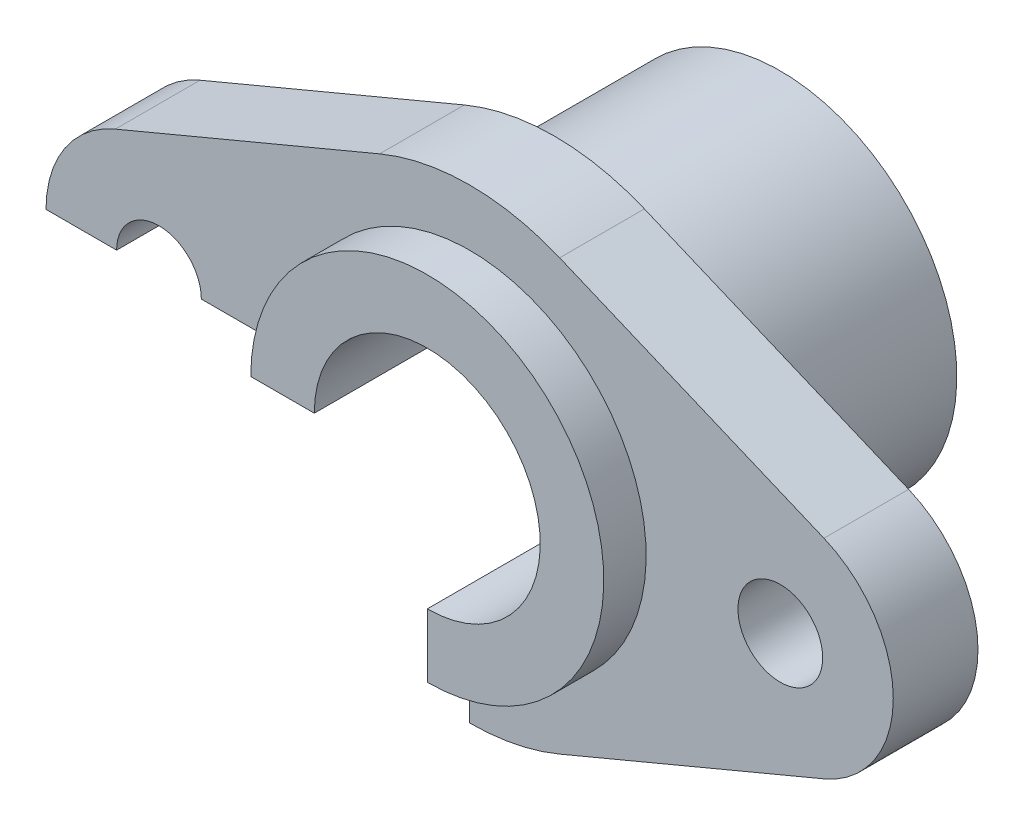
ISO-10303-21;
HEADER;
FILE_DESCRIPTION(('STEP AP214'),'2;1');
FILE_NAME('part.step','',(''),(''),'','','');
FILE_SCHEMA(('AUTOMOTIVE_DESIGN { 1 0 10303 214 1 1 1 1 }'));
ENDSEC;
DATA;
#1=APPLICATION_CONTEXT('core data for automotive mechanical design processes');
#2=APPLICATION_PROTOCOL_DEFINITION('international standard','automotive_design',2000,#1);
#3=PRODUCT_CONTEXT('',#1,'mechanical');
#4=PRODUCT('Part','Part','',(#3));
#5=PRODUCT_RELATED_PRODUCT_CATEGORY('part','',(#4));
#6=PRODUCT_DEFINITION_FORMATION('','',#4);
#7=PRODUCT_DEFINITION_CONTEXT('part definition',#1,'design');
#8=PRODUCT_DEFINITION('design','',#6,#7);
#9=PRODUCT_DEFINITION_SHAPE('','',#8);
#10=(LENGTH_UNIT() NAMED_UNIT(*) SI_UNIT(.MILLI.,.METRE.));
#11=(NAMED_UNIT(*) PLANE_ANGLE_UNIT() SI_UNIT($,.RADIAN.));
#12=(NAMED_UNIT(*) SI_UNIT($,.STERADIAN.) SOLID_ANGLE_UNIT());
#13=UNCERTAINTY_MEASURE_WITH_UNIT(LENGTH_MEASURE(1.E-05),#10,'distance_accuracy_value','');
#14=(GEOMETRIC_REPRESENTATION_CONTEXT(3) GLOBAL_UNCERTAINTY_ASSIGNED_CONTEXT((#13)) GLOBAL_UNIT_ASSIGNED_CONTEXT((#10,
#11,#12)) REPRESENTATION_CONTEXT('',''));
#15=CARTESIAN_POINT('',(0.,0.,0.));
#16=DIRECTION('',(0.,0.,1.));
#17=DIRECTION('',(1.,0.,0.));
#18=AXIS2_PLACEMENT_3D('',#15,#16,#17);
#19=CARTESIAN_POINT('',(-44.,0.,6.));
#20=DIRECTION('',(0.,0.,-1.));
#21=DIRECTION('',(-1.,0.,0.));
#22=AXIS2_PLACEMENT_3D('',#19,#20,#21);
#23=PLANE('',#22);
#24=CARTESIAN_POINT('',(-44.,0.,6.));
#25=DIRECTION('',(0.,0.,1.));
#26=DIRECTION('',(-1.,0.,0.));
#27=AXIS2_PLACEMENT_3D('',#24,#25,#26);
#28=CIRCLE('',#27,16.);
#29=CARTESIAN_POINT('',(-50.1818181818182,14.7575446456022,6.));
#30=VERTEX_POINT('',#29);
#31=CARTESIAN_POINT('',(-60.,0.,6.));
#32=VERTEX_POINT('',#31);
#33=EDGE_CURVE('E204',#30,#32,#28,.T.);
#34=ORIENTED_EDGE('',*,*,#33,.T.);
#35=DIRECTION('',(1.,0.,0.));
#36=VECTOR('',#35,1.);
#37=CARTESIAN_POINT('',(-44.,0.,6.));
#38=LINE('',#37,#36);
#39=CARTESIAN_POINT('',(-50.,0.,6.));
#40=VERTEX_POINT('',#39);
#41=EDGE_CURVE('E283',#32,#40,#38,.T.);
#42=ORIENTED_EDGE('',*,*,#41,.T.);
#43=CARTESIAN_POINT('',(-44.,0.,6.));
#44=DIRECTION('',(0.,0.,1.));
#45=DIRECTION('',(1.,0.,0.));
#46=AXIS2_PLACEMENT_3D('',#43,#44,#45);
#47=CIRCLE('',#46,6.);
#48=CARTESIAN_POINT('',(-38.,0.,6.));
#49=VERTEX_POINT('',#48);
#50=EDGE_CURVE('E196',#49,#40,#47,.T.);
#51=ORIENTED_EDGE('',*,*,#50,.F.);
#52=CARTESIAN_POINT('',(-25.,0.,6.));
#53=VERTEX_POINT('',#52);
#54=EDGE_CURVE('E280',#49,#53,#38,.T.);
#55=ORIENTED_EDGE('',*,*,#54,.T.);
#56=CARTESIAN_POINT('',(0.,0.,6.));
#57=DIRECTION('',(0.,0.,-1.));
#58=DIRECTION('',(-1.,0.,0.));
#59=AXIS2_PLACEMENT_3D('',#56,#57,#58);
#60=CIRCLE('',#59,25.);
#61=CARTESIAN_POINT('',(0.,-25.,6.));
#62=VERTEX_POINT('',#61);
#63=EDGE_CURVE('E185',#53,#62,#60,.T.);
#64=ORIENTED_EDGE('',*,*,#63,.T.);
#65=DIRECTION('',(0.,-1.,0.));
#66=VECTOR('',#65,1.);
#67=CARTESIAN_POINT('',(0.,0.,6.));
#68=LINE('',#67,#66);
#69=CARTESIAN_POINT('',(0.,-33.,6.));
#70=VERTEX_POINT('',#69);
#71=EDGE_CURVE('E275',#62,#70,#68,.T.);
#72=ORIENTED_EDGE('',*,*,#71,.T.);
#73=CARTESIAN_POINT('',(0.,0.,6.));
#74=DIRECTION('',(0.,0.,1.));
#75=DIRECTION('',(1.,0.,0.));
#76=AXIS2_PLACEMENT_3D('',#73,#74,#75);
#77=CIRCLE('',#76,33.);
#78=CARTESIAN_POINT('',(12.75,-30.4374358315545,6.));
#79=VERTEX_POINT('',#78);
#80=EDGE_CURVE('E210',#70,#79,#77,.T.);
#81=ORIENTED_EDGE('',*,*,#80,.T.);
#82=DIRECTION('',(0.922346540350137,0.386363636363636,0.));
#83=VECTOR('',#82,1.);
#84=CARTESIAN_POINT('',(12.75,-30.4374358315545,6.));
#85=LINE('',#84,#83);
#86=CARTESIAN_POINT('',(50.1818181818182,-14.7575446456022,6.));
#87=VERTEX_POINT('',#86);
#88=EDGE_CURVE('E209',#79,#87,#85,.T.);
#89=ORIENTED_EDGE('',*,*,#88,.T.);
#90=CARTESIAN_POINT('',(44.,0.,6.));
#91=DIRECTION('',(0.,0.,1.));
#92=DIRECTION('',(1.,0.,0.));
#93=AXIS2_PLACEMENT_3D('',#90,#91,#92);
#94=CIRCLE('',#93,16.);
#95=CARTESIAN_POINT('',(50.1818181818182,14.7575446456022,6.));
#96=VERTEX_POINT('',#95);
#97=EDGE_CURVE('E215',#87,#96,#94,.T.);
#98=ORIENTED_EDGE('',*,*,#97,.T.);
#99=DIRECTION('',(-0.922346540350137,0.386363636363636,0.));
#100=VECTOR('',#99,1.);
#101=CARTESIAN_POINT('',(12.75,30.4374358315545,6.));
#102=LINE('',#101,#100);
#103=CARTESIAN_POINT('',(12.75,30.4374358315545,6.));
#104=VERTEX_POINT('',#103);
#105=EDGE_CURVE('E212',#96,#104,#102,.T.);
#106=ORIENTED_EDGE('',*,*,#105,.T.);
#107=CARTESIAN_POINT('',(0.,0.,6.));
#108=DIRECTION('',(0.,0.,1.));
#109=DIRECTION('',(1.,0.,0.));
#110=AXIS2_PLACEMENT_3D('',#107,#108,#109);
#111=CIRCLE('',#110,33.);
#112=CARTESIAN_POINT('',(-12.75,30.4374358315545,6.));
#113=VERTEX_POINT('',#112);
#114=EDGE_CURVE('E216',#104,#113,#111,.T.);
#115=ORIENTED_EDGE('',*,*,#114,.T.);
#116=DIRECTION('',(-0.922346540350137,-0.386363636363636,0.));
#117=VECTOR('',#116,1.);
#118=CARTESIAN_POINT('',(-12.75,30.4374358315545,6.));
#119=LINE('',#118,#117);
#120=EDGE_CURVE('E217',#113,#30,#119,.T.);
#121=ORIENTED_EDGE('',*,*,#120,.T.);
#122=EDGE_LOOP('',(#34,#42,#51,#55,#64,#72,#81,#89,#98,#106,#115,#121));
#123=FACE_BOUND('',#122,.T.);
#124=CARTESIAN_POINT('',(44.,0.,6.));
#125=DIRECTION('',(0.,0.,1.));
#126=DIRECTION('',(1.,0.,0.));
#127=AXIS2_PLACEMENT_3D('',#124,#125,#126);
#128=CIRCLE('',#127,6.);
#129=CARTESIAN_POINT('',(50.,0.,6.));
#130=VERTEX_POINT('',#129);
#131=EDGE_CURVE('E195',#130,#130,#128,.T.);
#132=ORIENTED_EDGE('',*,*,#131,.F.);
#133=EDGE_LOOP('',(#132));
#134=FACE_BOUND('',#133,.T.);
#135=ADVANCED_FACE('F44',(#123,#134),#23,.F.);
#136=CARTESIAN_POINT('',(-44.,0.,-6.));
#137=DIRECTION('',(0.,0.,-1.));
#138=DIRECTION('',(-1.,0.,0.));
#139=AXIS2_PLACEMENT_3D('',#136,#137,#138);
#140=PLANE('',#139);
#141=DIRECTION('',(1.,0.,0.));
#142=VECTOR('',#141,1.);
#143=CARTESIAN_POINT('',(-44.,0.,-6.));
#144=LINE('',#143,#142);
#145=CARTESIAN_POINT('',(-60.,0.,-6.));
#146=VERTEX_POINT('',#145);
#147=CARTESIAN_POINT('',(-50.,0.,-6.));
#148=VERTEX_POINT('',#147);
#149=EDGE_CURVE('E58',#146,#148,#144,.T.);
#150=ORIENTED_EDGE('',*,*,#149,.F.);
#151=CARTESIAN_POINT('',(-44.,0.,-6.));
#152=DIRECTION('',(0.,0.,1.));
#153=DIRECTION('',(-1.,0.,0.));
#154=AXIS2_PLACEMENT_3D('',#151,#152,#153);
#155=CIRCLE('',#154,16.);
#156=CARTESIAN_POINT('',(-50.1818181818182,14.7575446456022,-6.));
#157=VERTEX_POINT('',#156);
#158=EDGE_CURVE('E203',#157,#146,#155,.T.);
#159=ORIENTED_EDGE('',*,*,#158,.F.);
#160=DIRECTION('',(-0.922346540350137,-0.386363636363636,0.));
#161=VECTOR('',#160,1.);
#162=CARTESIAN_POINT('',(-12.75,30.4374358315545,-6.));
#163=LINE('',#162,#161);
#164=CARTESIAN_POINT('',(-12.75,30.4374358315545,-6.));
#165=VERTEX_POINT('',#164);
#166=EDGE_CURVE('E208',#165,#157,#163,.T.);
#167=ORIENTED_EDGE('',*,*,#166,.F.);
#168=CARTESIAN_POINT('',(0.,0.,-6.));
#169=DIRECTION('',(0.,0.,1.));
#170=DIRECTION('',(1.,0.,0.));
#171=AXIS2_PLACEMENT_3D('',#168,#169,#170);
#172=CIRCLE('',#171,33.);
#173=CARTESIAN_POINT('',(12.75,30.4374358315545,-6.));
#174=VERTEX_POINT('',#173);
#175=EDGE_CURVE('E231',#174,#165,#172,.T.);
#176=ORIENTED_EDGE('',*,*,#175,.F.);
#177=DIRECTION('',(-0.922346540350137,0.386363636363636,0.));
#178=VECTOR('',#177,1.);
#179=CARTESIAN_POINT('',(12.75,30.4374358315545,-6.));
#180=LINE('',#179,#178);
#181=CARTESIAN_POINT('',(50.1818181818182,14.7575446456022,-6.));
#182=VERTEX_POINT('',#181);
#183=EDGE_CURVE('E230',#182,#174,#180,.T.);
#184=ORIENTED_EDGE('',*,*,#183,.F.);
#185=CARTESIAN_POINT('',(44.,0.,-6.));
#186=DIRECTION('',(0.,0.,1.));
#187=DIRECTION('',(1.,0.,0.));
#188=AXIS2_PLACEMENT_3D('',#185,#186,#187);
#189=CIRCLE('',#188,16.);
#190=CARTESIAN_POINT('',(50.1818181818182,-14.7575446456022,-6.));
#191=VERTEX_POINT('',#190);
#192=EDGE_CURVE('E229',#191,#182,#189,.T.);
#193=ORIENTED_EDGE('',*,*,#192,.F.);
#194=DIRECTION('',(0.922346540350137,0.386363636363636,0.));
#195=VECTOR('',#194,1.);
#196=CARTESIAN_POINT('',(12.75,-30.4374358315545,-6.));
#197=LINE('',#196,#195);
#198=CARTESIAN_POINT('',(12.75,-30.4374358315545,-6.));
#199=VERTEX_POINT('',#198);
#200=EDGE_CURVE('E223',#199,#191,#197,.T.);
#201=ORIENTED_EDGE('',*,*,#200,.F.);
#202=CARTESIAN_POINT('',(0.,0.,-6.));
#203=DIRECTION('',(0.,0.,1.));
#204=DIRECTION('',(1.,0.,0.));
#205=AXIS2_PLACEMENT_3D('',#202,#203,#204);
#206=CIRCLE('',#205,33.);
#207=CARTESIAN_POINT('',(0.,-33.,-6.));
#208=VERTEX_POINT('',#207);
#209=EDGE_CURVE('E224',#208,#199,#206,.T.);
#210=ORIENTED_EDGE('',*,*,#209,.F.);
#211=DIRECTION('',(0.,-1.,0.));
#212=VECTOR('',#211,1.);
#213=CARTESIAN_POINT('',(0.,0.,-6.));
#214=LINE('',#213,#212);
#215=CARTESIAN_POINT('',(0.,-25.,-6.));
#216=VERTEX_POINT('',#215);
#217=EDGE_CURVE('E266',#216,#208,#214,.T.);
#218=ORIENTED_EDGE('',*,*,#217,.F.);
#219=CARTESIAN_POINT('',(0.,0.,-6.));
#220=DIRECTION('',(0.,0.,-1.));
#221=DIRECTION('',(-1.,0.,0.));
#222=AXIS2_PLACEMENT_3D('',#219,#220,#221);
#223=CIRCLE('',#222,25.);
#224=CARTESIAN_POINT('',(-25.,0.,-6.));
#225=VERTEX_POINT('',#224);
#226=EDGE_CURVE('E253',#225,#216,#223,.T.);
#227=ORIENTED_EDGE('',*,*,#226,.F.);
#228=CARTESIAN_POINT('',(-38.,0.,-6.));
#229=VERTEX_POINT('',#228);
#230=EDGE_CURVE('E263',#229,#225,#144,.T.);
#231=ORIENTED_EDGE('',*,*,#230,.F.);
#232=CARTESIAN_POINT('',(-44.,0.,-6.));
#233=DIRECTION('',(0.,0.,1.));
#234=DIRECTION('',(1.,0.,0.));
#235=AXIS2_PLACEMENT_3D('',#232,#233,#234);
#236=CIRCLE('',#235,6.);
#237=EDGE_CURVE('E194',#229,#148,#236,.T.);
#238=ORIENTED_EDGE('',*,*,#237,.T.);
#239=EDGE_LOOP('',(#150,#159,#167,#176,#184,#193,#201,#210,#218,#227,#231,#238));
#240=FACE_BOUND('',#239,.T.);
#241=CARTESIAN_POINT('',(44.,0.,-6.));
#242=DIRECTION('',(0.,0.,1.));
#243=DIRECTION('',(1.,0.,0.));
#244=AXIS2_PLACEMENT_3D('',#241,#242,#243);
#245=CIRCLE('',#244,6.);
#246=CARTESIAN_POINT('',(50.,0.,-6.));
#247=VERTEX_POINT('',#246);
#248=EDGE_CURVE('E191',#247,#247,#245,.T.);
#249=ORIENTED_EDGE('',*,*,#248,.T.);
#250=EDGE_LOOP('',(#249));
#251=FACE_BOUND('',#250,.T.);
#252=ADVANCED_FACE('F261',(#240,#251),#140,.T.);
#253=CARTESIAN_POINT('',(-44.,0.,6.));
#254=DIRECTION('',(0.,0.,-1.));
#255=DIRECTION('',(-1.,0.,0.));
#256=AXIS2_PLACEMENT_3D('',#253,#254,#255);
#257=CYLINDRICAL_SURFACE('',#256,16.);
#258=ORIENTED_EDGE('',*,*,#158,.T.);
#259=DIRECTION('',(0.,0.,-1.));
#260=VECTOR('',#259,1.);
#261=CARTESIAN_POINT('',(-60.,0.,6.));
#262=LINE('',#261,#260);
#263=EDGE_CURVE('E287',#146,#32,#262,.F.);
#264=ORIENTED_EDGE('',*,*,#263,.T.);
#265=ORIENTED_EDGE('',*,*,#33,.F.);
#266=DIRECTION('',(0.,0.,-1.));
#267=VECTOR('',#266,1.);
#268=CARTESIAN_POINT('',(-50.1818181818182,14.7575446456022,6.));
#269=LINE('',#268,#267);
#270=EDGE_CURVE('E219',#30,#157,#269,.T.);
#271=ORIENTED_EDGE('',*,*,#270,.T.);
#272=EDGE_LOOP('',(#258,#264,#265,#271));
#273=FACE_BOUND('',#272,.T.);
#274=ADVANCED_FACE('F50',(#273),#257,.T.);
#275=CARTESIAN_POINT('',(0.,0.,6.));
#276=DIRECTION('',(0.,0.,-1.));
#277=DIRECTION('',(-1.,0.,0.));
#278=AXIS2_PLACEMENT_3D('',#275,#276,#277);
#279=CYLINDRICAL_SURFACE('',#278,33.);
#280=ORIENTED_EDGE('',*,*,#80,.F.);
#281=DIRECTION('',(0.,0.,-1.));
#282=VECTOR('',#281,1.);
#283=CARTESIAN_POINT('',(0.,-33.,6.));
#284=LINE('',#283,#282);
#285=EDGE_CURVE('E267',#70,#208,#284,.T.);
#286=ORIENTED_EDGE('',*,*,#285,.T.);
#287=ORIENTED_EDGE('',*,*,#209,.T.);
#288=DIRECTION('',(0.,0.,-1.));
#289=VECTOR('',#288,1.);
#290=CARTESIAN_POINT('',(12.75,-30.4374358315545,6.));
#291=LINE('',#290,#289);
#292=EDGE_CURVE('E247',#79,#199,#291,.T.);
#293=ORIENTED_EDGE('',*,*,#292,.F.);
#294=EDGE_LOOP('',(#280,#286,#287,#293));
#295=FACE_BOUND('',#294,.T.);
#296=ADVANCED_FACE('F337',(#295),#279,.T.);
#297=CARTESIAN_POINT('',(12.75,-30.4374358315545,6.));
#298=DIRECTION('',(-0.386363636363636,0.922346540350137,0.));
#299=DIRECTION('',(-0.922346540350138,-0.386363636363637,0.));
#300=AXIS2_PLACEMENT_3D('',#297,#298,#299);
#301=PLANE('',#300);
#302=ORIENTED_EDGE('',*,*,#200,.T.);
#303=DIRECTION('',(0.,0.,-1.));
#304=VECTOR('',#303,1.);
#305=CARTESIAN_POINT('',(50.1818181818182,-14.7575446456022,6.));
#306=LINE('',#305,#304);
#307=EDGE_CURVE('E241',#87,#191,#306,.T.);
#308=ORIENTED_EDGE('',*,*,#307,.F.);
#309=ORIENTED_EDGE('',*,*,#88,.F.);
#310=ORIENTED_EDGE('',*,*,#292,.T.);
#311=EDGE_LOOP('',(#302,#308,#309,#310));
#312=FACE_BOUND('',#311,.T.);
#313=ADVANCED_FACE('F331',(#312),#301,.F.);
#314=CARTESIAN_POINT('',(44.,0.,6.));
#315=DIRECTION('',(0.,0.,-1.));
#316=DIRECTION('',(-1.,0.,0.));
#317=AXIS2_PLACEMENT_3D('',#314,#315,#316);
#318=CYLINDRICAL_SURFACE('',#317,16.);
#319=ORIENTED_EDGE('',*,*,#192,.T.);
#320=DIRECTION('',(0.,0.,-1.));
#321=VECTOR('',#320,1.);
#322=CARTESIAN_POINT('',(50.1818181818182,14.7575446456022,6.));
#323=LINE('',#322,#321);
#324=EDGE_CURVE('E244',#96,#182,#323,.T.);
#325=ORIENTED_EDGE('',*,*,#324,.F.);
#326=ORIENTED_EDGE('',*,*,#97,.F.);
#327=ORIENTED_EDGE('',*,*,#307,.T.);
#328=EDGE_LOOP('',(#319,#325,#326,#327));
#329=FACE_BOUND('',#328,.T.);
#330=ADVANCED_FACE('F332',(#329),#318,.T.);
#331=CARTESIAN_POINT('',(12.75,30.4374358315545,6.));
#332=DIRECTION('',(-0.386363636363636,-0.922346540350137,0.));
#333=DIRECTION('',(0.922346540350138,-0.386363636363637,0.));
#334=AXIS2_PLACEMENT_3D('',#331,#332,#333);
#335=PLANE('',#334);
#336=ORIENTED_EDGE('',*,*,#183,.T.);
#337=DIRECTION('',(0.,0.,-1.));
#338=VECTOR('',#337,1.);
#339=CARTESIAN_POINT('',(12.75,30.4374358315545,6.));
#340=LINE('',#339,#338);
#341=EDGE_CURVE('E239',#104,#174,#340,.T.);
#342=ORIENTED_EDGE('',*,*,#341,.F.);
#343=ORIENTED_EDGE('',*,*,#105,.F.);
#344=ORIENTED_EDGE('',*,*,#324,.T.);
#345=EDGE_LOOP('',(#336,#342,#343,#344));
#346=FACE_BOUND('',#345,.T.);
#347=ADVANCED_FACE('F330',(#346),#335,.F.);
#348=CARTESIAN_POINT('',(0.,0.,6.));
#349=DIRECTION('',(0.,0.,-1.));
#350=DIRECTION('',(-1.,0.,0.));
#351=AXIS2_PLACEMENT_3D('',#348,#349,#350);
#352=CYLINDRICAL_SURFACE('',#351,33.);
#353=ORIENTED_EDGE('',*,*,#175,.T.);
#354=DIRECTION('',(0.,0.,-1.));
#355=VECTOR('',#354,1.);
#356=CARTESIAN_POINT('',(-12.75,30.4374358315545,6.));
#357=LINE('',#356,#355);
#358=EDGE_CURVE('E237',#113,#165,#357,.T.);
#359=ORIENTED_EDGE('',*,*,#358,.F.);
#360=ORIENTED_EDGE('',*,*,#114,.F.);
#361=ORIENTED_EDGE('',*,*,#341,.T.);
#362=EDGE_LOOP('',(#353,#359,#360,#361));
#363=FACE_BOUND('',#362,.T.);
#364=ADVANCED_FACE('F325',(#363),#352,.T.);
#365=CARTESIAN_POINT('',(-12.75,30.4374358315545,6.));
#366=DIRECTION('',(0.386363636363636,-0.922346540350137,0.));
#367=DIRECTION('',(0.922346540350138,0.386363636363637,0.));
#368=AXIS2_PLACEMENT_3D('',#365,#366,#367);
#369=PLANE('',#368);
#370=ORIENTED_EDGE('',*,*,#166,.T.);
#371=ORIENTED_EDGE('',*,*,#270,.F.);
#372=ORIENTED_EDGE('',*,*,#120,.F.);
#373=ORIENTED_EDGE('',*,*,#358,.T.);
#374=EDGE_LOOP('',(#370,#371,#372,#373));
#375=FACE_BOUND('',#374,.T.);
#376=ADVANCED_FACE('F316',(#375),#369,.F.);
#377=CARTESIAN_POINT('',(-44.,0.,6.));
#378=DIRECTION('',(0.,0.,-1.));
#379=DIRECTION('',(-1.,0.,0.));
#380=AXIS2_PLACEMENT_3D('',#377,#378,#379);
#381=CYLINDRICAL_SURFACE('',#380,6.);
#382=DIRECTION('',(0.,0.,-1.));
#383=VECTOR('',#382,1.);
#384=CARTESIAN_POINT('',(-38.,0.,6.));
#385=LINE('',#384,#383);
#386=EDGE_CURVE('E278',#49,#229,#385,.T.);
#387=ORIENTED_EDGE('',*,*,#386,.F.);
#388=ORIENTED_EDGE('',*,*,#50,.T.);
#389=DIRECTION('',(0.,0.,-1.));
#390=VECTOR('',#389,1.);
#391=CARTESIAN_POINT('',(-50.,0.,6.));
#392=LINE('',#391,#390);
#393=EDGE_CURVE('E286',#148,#40,#392,.F.);
#394=ORIENTED_EDGE('',*,*,#393,.F.);
#395=ORIENTED_EDGE('',*,*,#237,.F.);
#396=EDGE_LOOP('',(#387,#388,#394,#395));
#397=FACE_BOUND('',#396,.T.);
#398=ADVANCED_FACE('F306',(#397),#381,.F.);
#399=CARTESIAN_POINT('',(44.,0.,6.));
#400=DIRECTION('',(0.,0.,-1.));
#401=DIRECTION('',(-1.,0.,0.));
#402=AXIS2_PLACEMENT_3D('',#399,#400,#401);
#403=CYLINDRICAL_SURFACE('',#402,6.);
#404=ORIENTED_EDGE('',*,*,#131,.T.);
#405=EDGE_LOOP('',(#404));
#406=FACE_BOUND('',#405,.T.);
#407=ORIENTED_EDGE('',*,*,#248,.F.);
#408=EDGE_LOOP('',(#407));
#409=FACE_BOUND('',#408,.T.);
#410=ADVANCED_FACE('F423',(#406,#409),#403,.F.);
#411=CARTESIAN_POINT('',(0.,0.,-38.));
#412=DIRECTION('',(0.,0.,1.));
#413=DIRECTION('',(1.,0.,0.));
#414=AXIS2_PLACEMENT_3D('',#411,#412,#413);
#415=CYLINDRICAL_SURFACE('',#414,25.);
#416=DIRECTION('',(0.,0.,1.));
#417=VECTOR('',#416,1.);
#418=CARTESIAN_POINT('',(-25.,0.,-38.));
#419=LINE('',#418,#417);
#420=CARTESIAN_POINT('',(-25.,0.,-38.));
#421=VERTEX_POINT('',#420);
#422=EDGE_CURVE('E260',#225,#421,#419,.F.);
#423=ORIENTED_EDGE('',*,*,#422,.F.);
#424=ORIENTED_EDGE('',*,*,#226,.T.);
#425=DIRECTION('',(0.,0.,1.));
#426=VECTOR('',#425,1.);
#427=CARTESIAN_POINT('',(0.,-25.,-38.));
#428=LINE('',#427,#426);
#429=CARTESIAN_POINT('',(0.,-25.,-38.));
#430=VERTEX_POINT('',#429);
#431=EDGE_CURVE('E170',#430,#216,#428,.T.);
#432=ORIENTED_EDGE('',*,*,#431,.F.);
#433=CARTESIAN_POINT('',(0.,0.,-38.));
#434=DIRECTION('',(0.,0.,1.));
#435=DIRECTION('',(1.,0.,0.));
#436=AXIS2_PLACEMENT_3D('',#433,#434,#435);
#437=CIRCLE('',#436,25.);
#438=EDGE_CURVE('E176',#430,#421,#437,.T.);
#439=ORIENTED_EDGE('',*,*,#438,.T.);
#440=EDGE_LOOP('',(#423,#424,#432,#439));
#441=FACE_BOUND('',#440,.T.);
#442=ADVANCED_FACE('F258',(#441),#415,.T.);
#443=CARTESIAN_POINT('',(0.,0.,-38.));
#444=DIRECTION('',(0.,0.,1.));
#445=DIRECTION('',(1.,0.,0.));
#446=AXIS2_PLACEMENT_3D('',#443,#444,#445);
#447=PLANE('',#446);
#448=CARTESIAN_POINT('',(0.,0.,-38.));
#449=DIRECTION('',(0.,0.,1.));
#450=DIRECTION('',(1.,0.,0.));
#451=AXIS2_PLACEMENT_3D('',#448,#449,#450);
#452=CIRCLE('',#451,16.);
#453=CARTESIAN_POINT('',(0.,-16.,-38.));
#454=VERTEX_POINT('',#453);
#455=CARTESIAN_POINT('',(-16.,0.,-38.));
#456=VERTEX_POINT('',#455);
#457=EDGE_CURVE('E175',#454,#456,#452,.T.);
#458=ORIENTED_EDGE('',*,*,#457,.T.);
#459=DIRECTION('',(1.,0.,0.));
#460=VECTOR('',#459,1.);
#461=CARTESIAN_POINT('',(-30.8294609287128,0.,-38.));
#462=LINE('',#461,#460);
#463=EDGE_CURVE('E180',#421,#456,#462,.T.);
#464=ORIENTED_EDGE('',*,*,#463,.F.);
#465=ORIENTED_EDGE('',*,*,#438,.F.);
#466=DIRECTION('',(0.,-1.,0.));
#467=VECTOR('',#466,1.);
#468=CARTESIAN_POINT('',(0.,-48.6211784165391,-38.));
#469=LINE('',#468,#467);
#470=EDGE_CURVE('E157',#454,#430,#469,.T.);
#471=ORIENTED_EDGE('',*,*,#470,.F.);
#472=EDGE_LOOP('',(#458,#464,#465,#471));
#473=FACE_BOUND('',#472,.T.);
#474=ADVANCED_FACE('F174',(#473),#447,.F.);
#475=CARTESIAN_POINT('',(0.,0.,-6.));
#476=DIRECTION('',(0.,0.,1.));
#477=DIRECTION('',(1.,0.,0.));
#478=AXIS2_PLACEMENT_3D('',#475,#476,#477);
#479=CYLINDRICAL_SURFACE('',#478,16.);
#480=CARTESIAN_POINT('',(0.,0.,12.));
#481=DIRECTION('',(0.,0.,1.));
#482=DIRECTION('',(1.,0.,0.));
#483=AXIS2_PLACEMENT_3D('',#480,#481,#482);
#484=CIRCLE('',#483,16.);
#485=CARTESIAN_POINT('',(0.,-16.,12.));
#486=VERTEX_POINT('',#485);
#487=CARTESIAN_POINT('',(-16.,0.,12.));
#488=VERTEX_POINT('',#487);
#489=EDGE_CURVE('E183',#486,#488,#484,.T.);
#490=ORIENTED_EDGE('',*,*,#489,.T.);
#491=DIRECTION('',(0.,0.,1.));
#492=VECTOR('',#491,1.);
#493=CARTESIAN_POINT('',(-16.,0.,-6.));
#494=LINE('',#493,#492);
#495=EDGE_CURVE('E70',#488,#456,#494,.F.);
#496=ORIENTED_EDGE('',*,*,#495,.T.);
#497=ORIENTED_EDGE('',*,*,#457,.F.);
#498=DIRECTION('',(0.,0.,1.));
#499=VECTOR('',#498,1.);
#500=CARTESIAN_POINT('',(0.,-16.,-6.));
#501=LINE('',#500,#499);
#502=EDGE_CURVE('E156',#454,#486,#501,.T.);
#503=ORIENTED_EDGE('',*,*,#502,.T.);
#504=EDGE_LOOP('',(#490,#496,#497,#503));
#505=FACE_BOUND('',#504,.T.);
#506=ADVANCED_FACE('F178',(#505),#479,.F.);
#507=DIRECTION('',(0.,0.,1.));
#508=VECTOR('',#507,1.);
#509=CARTESIAN_POINT('',(-25.,0.,-38.));
#510=LINE('',#509,#508);
#511=CARTESIAN_POINT('',(-25.,0.,12.));
#512=VERTEX_POINT('',#511);
#513=EDGE_CURVE('E167',#512,#53,#510,.F.);
#514=ORIENTED_EDGE('',*,*,#513,.F.);
#515=CARTESIAN_POINT('',(0.,0.,12.));
#516=DIRECTION('',(0.,0.,1.));
#517=DIRECTION('',(1.,0.,0.));
#518=AXIS2_PLACEMENT_3D('',#515,#516,#517);
#519=CIRCLE('',#518,25.);
#520=CARTESIAN_POINT('',(0.,-25.,12.));
#521=VERTEX_POINT('',#520);
#522=EDGE_CURVE('E179',#521,#512,#519,.T.);
#523=ORIENTED_EDGE('',*,*,#522,.F.);
#524=DIRECTION('',(0.,0.,1.));
#525=VECTOR('',#524,1.);
#526=CARTESIAN_POINT('',(0.,-25.,-38.));
#527=LINE('',#526,#525);
#528=EDGE_CURVE('E300',#62,#521,#527,.T.);
#529=ORIENTED_EDGE('',*,*,#528,.F.);
#530=ORIENTED_EDGE('',*,*,#63,.F.);
#531=EDGE_LOOP('',(#514,#523,#529,#530));
#532=FACE_BOUND('',#531,.T.);
#533=ADVANCED_FACE('F299',(#532),#415,.T.);
#534=CARTESIAN_POINT('',(0.,0.,12.));
#535=DIRECTION('',(0.,0.,1.));
#536=DIRECTION('',(1.,0.,0.));
#537=AXIS2_PLACEMENT_3D('',#534,#535,#536);
#538=PLANE('',#537);
#539=DIRECTION('',(-1.,0.,0.));
#540=VECTOR('',#539,1.);
#541=CARTESIAN_POINT('',(0.,0.,12.));
#542=LINE('',#541,#540);
#543=EDGE_CURVE('E11',#488,#512,#542,.T.);
#544=ORIENTED_EDGE('',*,*,#543,.F.);
#545=ORIENTED_EDGE('',*,*,#489,.F.);
#546=DIRECTION('',(0.,1.,0.));
#547=VECTOR('',#546,1.);
#548=CARTESIAN_POINT('',(0.,0.,12.));
#549=LINE('',#548,#547);
#550=EDGE_CURVE('E52',#521,#486,#549,.T.);
#551=ORIENTED_EDGE('',*,*,#550,.F.);
#552=ORIENTED_EDGE('',*,*,#522,.T.);
#553=EDGE_LOOP('',(#544,#545,#551,#552));
#554=FACE_BOUND('',#553,.T.);
#555=ADVANCED_FACE('F292',(#554),#538,.T.);
#556=CARTESIAN_POINT('',(0.,-48.6211784165391,12.));
#557=DIRECTION('',(1.,0.,0.));
#558=DIRECTION('',(0.,0.,-1.));
#559=AXIS2_PLACEMENT_3D('',#556,#557,#558);
#560=PLANE('',#559);
#561=ORIENTED_EDGE('',*,*,#470,.T.);
#562=ORIENTED_EDGE('',*,*,#431,.T.);
#563=ORIENTED_EDGE('',*,*,#217,.T.);
#564=ORIENTED_EDGE('',*,*,#285,.F.);
#565=ORIENTED_EDGE('',*,*,#71,.F.);
#566=ORIENTED_EDGE('',*,*,#528,.T.);
#567=ORIENTED_EDGE('',*,*,#550,.T.);
#568=ORIENTED_EDGE('',*,*,#502,.F.);
#569=EDGE_LOOP('',(#561,#562,#563,#564,#565,#566,#567,#568));
#570=FACE_BOUND('',#569,.T.);
#571=ADVANCED_FACE('F158',(#570),#560,.F.);
#572=CARTESIAN_POINT('',(-30.8294609287128,0.,12.));
#573=DIRECTION('',(0.,1.,0.));
#574=DIRECTION('',(0.,0.,1.));
#575=AXIS2_PLACEMENT_3D('',#572,#573,#574);
#576=PLANE('',#575);
#577=ORIENTED_EDGE('',*,*,#543,.T.);
#578=ORIENTED_EDGE('',*,*,#513,.T.);
#579=ORIENTED_EDGE('',*,*,#54,.F.);
#580=ORIENTED_EDGE('',*,*,#386,.T.);
#581=ORIENTED_EDGE('',*,*,#230,.T.);
#582=ORIENTED_EDGE('',*,*,#422,.T.);
#583=ORIENTED_EDGE('',*,*,#463,.T.);
#584=ORIENTED_EDGE('',*,*,#495,.F.);
#585=EDGE_LOOP('',(#577,#578,#579,#580,#581,#582,#583,#584));
#586=FACE_BOUND('',#585,.T.);
#587=ADVANCED_FACE('F294',(#586),#576,.F.);
#588=ORIENTED_EDGE('',*,*,#149,.T.);
#589=ORIENTED_EDGE('',*,*,#393,.T.);
#590=ORIENTED_EDGE('',*,*,#41,.F.);
#591=ORIENTED_EDGE('',*,*,#263,.F.);
#592=EDGE_LOOP('',(#588,#589,#590,#591));
#593=FACE_BOUND('',#592,.T.);
#594=ADVANCED_FACE('F341',(#593),#576,.F.);
#595=CLOSED_SHELL('',(#135,#252,#274,#296,#313,#330,#347,#364,#376,#398,#410,#442,#474,#506,
#533,#555,#571,#587,#594));
#596=MANIFOLD_SOLID_BREP('B2',#595);
#597=ADVANCED_BREP_SHAPE_REPRESENTATION('',(#18,#596),#14);
#598=SHAPE_DEFINITION_REPRESENTATION(#9,#597);
ENDSEC;
END-ISO-10303-21;
